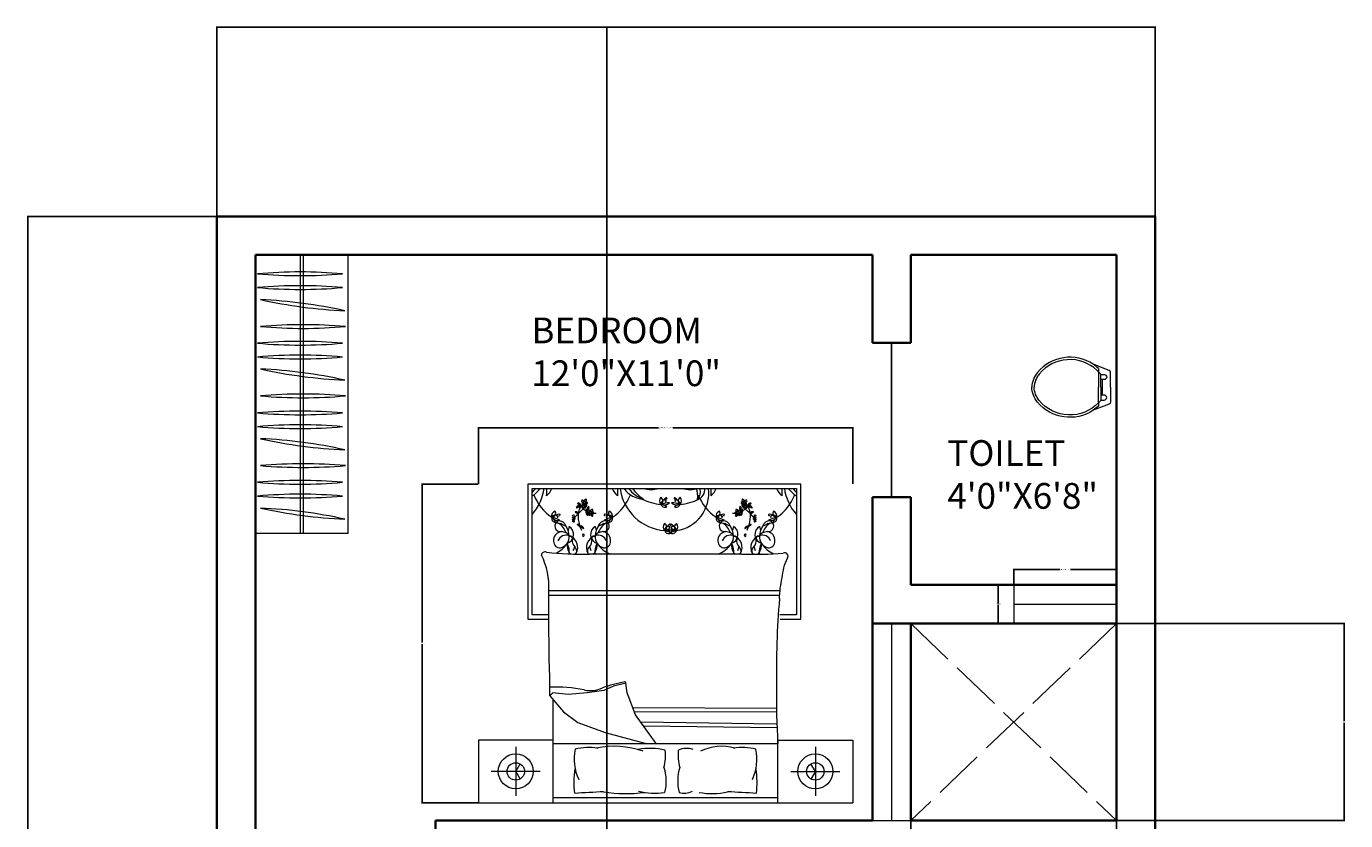
# Model space of a CAD drawing. Units: inches. Extents: x -16 to 587, y -783 to 64.
# Tile 14 of 14: x 279 to 587, y -122 to 64. Entities that reach past the tile are written whole.
import ezdxf

# ---------------------------------------------------------------- set-up
doc = ezdxf.new("R2010")
doc.units = ezdxf.units.IN
doc.header["$MEASUREMENT"] = 0
doc.linetypes.add('ACAD_ISO02W100', pattern=[15, 12, -3])
for name, color, linetype, lineweight in [('A-ANNO-DIMS', 2, 'Continuous', 18), ('A-AREA-IDEN', 7, 'Continuous', 18), ('A-DOOR', 3, 'Continuous', 25), ('A-FLOR-FIXT', 9, 'Continuous', 18), ('A-FLOR-OPEN', 8, 'ACAD_ISO02W100', 13), ('A-FURN', 8, 'Continuous', 18), ('A-GLAZ', 4, 'Continuous', 18), ('A-WALL', 7, 'Continuous', 35)]:
    doc.layers.add(name, color=color, linetype=linetype, lineweight=lineweight)
doc.styles.get("Standard").update_dxf_attribs({"font": 'arial.ttf'})
doc.dimstyles.get("Standard").update_dxf_attribs({"dimtxt": 0.18, "dimasz": 0.18, "dimexe": 0.18, "dimexo": 0.0625, "dimgap": 0.09, "dimtad": 0, "dimtih": 1, "dimtoh": 1, "dimdec": 0, "dimzin": 0, "dimdsep": 46, "dimlunit": 3, "dimtxsty": 'Standard', "dimcen": 0.09, "dimadec": 0, "dimazin": 0, "dimtfac": 1, "dimtdec": 0, "dimtofl": 0, "dimtmove": 0, "dimatfit": 3, "dimfxl": 1, "dimtolj": 1, "dimtzin": 0, "dimarcsym": 0})

# ---------------------------------------------------------------- blocks, each defined once
blk = doc.blocks.new('BED-DOUBLE-LARGE')
for p, q in [((11.54, 74.35), (11.54, 42.86)), ((75.28, 74.35), (11.54, 74.35)), ((75.28, 42.86), (75.28, 74.35)), ((12.55, 73.34), (74.26, 73.34)), ((12.55, 43.87), (12.55, 73.34)), ((74.26, 73.34), (74.26, 43.87)), ((21.17, 64.47), (20.98, 63.49)), ((27.28, 64.47), (27.47, 63.49)), ((59.54, 64.47), (59.35, 63.49)), ((65.65, 64.47), (65.84, 63.49)), ((61.46, 57.99), (25.97, 57.99)), ((70.42, 49.4), (16.48, 49.4)), ((70.34, 48.31), (16.48, 48.31)), ((16.48, 43.87), (12.55, 43.87)), ((74.26, 43.87), (70.41, 43.87)), ((11.54, 42.86), (16.49, 42.86)), ((70.43, 42.86), (75.28, 42.86)), ((34.41, 27.92), (31.58, 27.21)), ((34.77, 25.62), (34.41, 27.92)), ((17.41, 25.62), (16.7, 24.91)), ((16.7, 24.91), (19.89, 21.19)), ((20.95, 25.26), (17.41, 25.62)), ((25.38, 25.62), (20.95, 25.26)), ((29.28, 26.15), (25.38, 25.62)), ((31.58, 27.21), (29.28, 26.15)), ((36.71, 20.49), (34.77, 25.62)), ((17.49, 0), (17.49, 24)), ((69.63, 22), (36.09, 22.13)), ((19.89, 21.19), (23.25, 18.72)), ((23.25, 18.72), (29.63, 16.41)), ((69.63, 21.1), (36.43, 21.23)), ((41.5, 13.82), (36.71, 20.49)), ((69.67, 18.35), (37.93, 18.79)), ((29.63, 16.41), (39.16, 13.82)), ((69.71, 17.45), (38.58, 17.88)), ((8.74, 13), (8.74, 1.57)), ((17.49, 13.82), (69.94, 13.82)), ((78.68, 13), (78.68, 1.57)), ((14.46, 7.29), (3.03, 7.29)), ((72.97, 7.29), (84.4, 7.29)), ((0, 0), (87.43, 0)), ((69.94, 1.12), (17.49, 1.12))]:
    blk.add_line(p, q)
for points in [[(16.52, 32.91, -0.001242), (16.48, 49.5, 0.127202), (14.73, 57.77)], [(70.32, 47.62, -0.056112), (70.95, 52.43, -0.095341), (72.18, 57.07)], [(22.51, 2.18, -0.074897), (22.61, 7.89, 0.472817)], [(43.3, 8.21, -0.14099), (43.48, 2.38, -0.235245)], [(47.04, 8.21, 0.14099), (46.86, 2.38, 0.235245)], [(64.92, 2.18, 0.074897), (64.81, 7.89, -0.472817)]]:
    blk.add_lwpolyline(points, format="xyb")
for points in [[(17.49, 14.57), (0, 14.57), (0, 0)], [(69.94, 0), (69.94, 14.57), (87.43, 14.57), (87.43, 0)], [(8.74, 7.29), (9.76, 9.05)], [(8.74, 7.29), (9.76, 5.52)], [(78.68, 7.29), (77.66, 9.05)], [(78.68, 7.29), (77.66, 5.52)]]:
    blk.add_lwpolyline(points)
for centre, radius in [((24.76, 69.99), 0.223), ((26.22, 67.64), 0.223), ((60.6, 67.64), 0.223), ((62.05, 69.99), 0.223), ((8.74, 7.29), 4.08), ((8.74, 7.29), 2.04), ((78.68, 7.29), 4.08), ((78.68, 7.29), 2.04)]:
    blk.add_circle(centre, radius)
for centre, radius, start, end in [((7.78, 77.44), 6.93, 313.5186, 323.6964), ((9.78, 76.41), 5.56, 299.8884, 326.5383), ((4.05, 74.88), 11.42, 318.1144, 352.255), ((23.59, 76.01), 11.42, 201.4092, 235.6135), ((12.9, 75.12), 4.64, 311.0454, 337.4453), ((0.18, 72.62), 15.8, 356.3481, 2.5919), ((35.55, 75.12), 4.64, 202.5547, 228.9546), ((24.86, 76.01), 11.42, 304.3865, 338.5908), ((48.27, 72.62), 15.8, 177.4081, 183.6519), ((44.39, 74.88), 11.42, 187.745, 265.5377), ((38.67, 76.41), 5.56, 213.4617, 268.728), ((40.67, 77.44), 6.93, 216.3036, 252.1496), ((44.31, 79.39), 10.31, 215.947, 235.9877), ((43.52, 80.99), 11.42, 242.5854, 265.5377), ((40.33, 79.34), 6.28, 252.9798, 286.4569), ((42.81, 82.58), 9.28, 264.3643, 265.6213), ((47.7, 88.94), 16.59, 250.0972, 250.2783), ((43.57, 70.46), 1.27, 140.8855, 222.2127), ((42.13, 70.42), 0.953, 301.6373, 61.4609), ((45.36, 68.67), 2.89, 121.989, 161.0841), ((43.91, 71), 0.142, 288.4408, 121.989), ((43.93, 70.93), 0.0689, 171.9833, 288.4408), ((45.82, 71), 0.142, 58.011, 251.5592), ((45.8, 70.93), 0.0689, 251.5592, 8.0167), ((44.37, 68.67), 2.89, 18.9159, 58.011), ((44.97, 72.24), 8.84, 278.1803, 7.1364), ((47.6, 70.42), 0.953, 118.5391, 238.3627), ((46.16, 70.46), 1.27, 317.7873, 39.1145), ((46.21, 80.99), 11.42, 274.4623, 297.4146), ((49.41, 79.34), 6.28, 253.5431, 287.0202), ((46.92, 82.58), 9.28, 274.3787, 275.6357), ((42.03, 88.94), 16.59, 289.7217, 289.9028), ((46.11, 71.43), 5.11, 353.3805, 21.883), ((50.8, 72.86), 2.05, 280.9261, 13.6102), ((49.26, 72.57), 2.59, 318.0951, 17.1391), ((61.96, 76.01), 11.42, 201.4092, 235.6135), ((38.55, 72.62), 15.8, 356.3481, 2.5919), ((51.27, 75.12), 4.64, 311.0454, 337.4453), ((73.92, 75.12), 4.64, 202.5547, 228.9546), ((63.23, 76.01), 11.42, 304.3865, 338.5908), ((86.64, 72.62), 15.8, 177.4081, 183.6519), ((82.76, 74.88), 11.42, 187.745, 221.8856), ((77.04, 76.41), 5.56, 213.4617, 240.1116), ((79.04, 77.44), 6.93, 216.3036, 226.4814), ((18.37, 66.85), 1.27, 110.9613, 192.2885), ((17.11, 67.54), 0.953, 271.7131, 31.5367), ((22.65, 65.38), 2.47, 82.8698, 91.6736), ((22.99, 68.05), 0.459, 205.5379, 258.6744), ((22.33, 66.49), 1.38, 59.344, 79.7412), ((23.14, 68.85), 0.249, 123.0979, 213.1364), ((23.57, 68.49), 0.673, 92.3172, 160.5201), ((26.65, 63.38), 6.5, 121.1156, 124.8118), ((22.89, 67.42), 0.42, 355.7131, 81.6568), ((23.49, 68.75), 0.58, 82.6008, 147.1845), ((23.33, 69.66), 0.249, 55.6077, 145.6462), ((23.16, 69.13), 0.673, 21.7087, 93.0299), ((19.61, 64.33), 6.5, 53.6254, 57.3216), ((23.42, 68.72), 0.257, 45.7354, 121.1156), ((26.93, 67.08), 3.63, 150.7959, 175.244), ((32.15, 59.35), 11.95, 127.8256, 137.7588), ((23.36, 69.3), 0.58, 342.8042, 79.6943), ((23.31, 69.36), 0.257, 338.2452, 53.6254), ((23.73, 69.19), 0.194, 158.2452, 340.6395), ((23.74, 69.05), 0.194, 225.7354, 48.1297), ((27.39, 70.82), 3.88, 201.7087, 206.2181), ((24.3, 68.17), 1.01, 40.9365, 112.7695), ((23.96, 68.51), 0.597, 49.3812, 95.5456), ((26.93, 67.08), 3.63, 137.5083, 145.9967), ((24.4, 68.75), 0.617, 61.1838, 141.6792), ((27.3, 71.9), 4.35, 220.182, 239.456), ((24.3, 70.41), 0.221, 134.3732, 211.9501), ((24.7, 70.66), 0.702, 211.9501, 255.2442), ((24.31, 70.16), 0.439, 8.5614, 112.5914), ((24.52, 69.68), 0.304, 88.5719, 233.8954), ((24.48, 69.6), 0.218, 228.2946, 6.2474), ((24.82, 69.51), 0.718, 229.3812, 289.9959), ((24.43, 70.18), 0.147, 352.868, 97.094), ((24.28, 69.86), 0.306, 298.8493, 359.9355), ((24.35, 69.6), 0.35, 4.2123, 48.1587), ((25.07, 70.4), 0.368, 100.9597, 208.7804), ((25.07, 69.64), 0.371, 183.635, 258.4363), ((24.36, 68.63), 0.737, 15.6484, 62.2957), ((25.02, 69.78), 0.213, 178.1325, 268.8919), ((25.46, 69.91), 0.676, 132.3896, 156.5724), ((25.17, 69.83), 0.364, 42.3208, 130.2111), ((25.25, 70.21), 0.46, 226.3462, 279.6513), ((24.77, 69.35), 0.535, 7.4968, 71.2737), ((24.76, 70.6), 0.517, 291.6382, 4.947), ((25.16, 70.68), 0.729, 254.2829, 276.9148), ((25.1, 70.63), 0.171, 4.947, 127.5263), ((25.14, 69.38), 0.172, 215.0752, 14.7644), ((24.78, 69.11), 1.01, 287.889, 359.722), ((24.75, 68.64), 0.597, 305.1128, 351.2773), ((25.06, 67.54), 0.617, 3.8774, 87.1501), ((24.62, 67.78), 0.597, 352.0748, 38.2393), ((24.52, 67.31), 1.01, 343.6301, 55.4631), ((25.23, 68.74), 0.617, 271.4625, 339.4747), ((25.29, 69.94), 0.192, 279.6513, 42.3208), ((26.05, 68.44), 0.718, 110.6625, 171.2773), ((25.75, 68.06), 0.221, 134.3732, 211.9501), ((27.3, 71.9), 4.35, 246.1523, 246.9499), ((26.16, 68.32), 0.702, 211.9501, 255.2442), ((25.77, 67.81), 0.439, 8.5614, 112.5914), ((25.13, 68.8), 0.737, 338.3627, 25.0101), ((25.89, 67.83), 0.147, 352.868, 97.094), ((26.52, 68.05), 0.368, 100.9597, 208.7804), ((26.92, 67.57), 0.676, 132.3896, 156.5724), ((26.62, 67.48), 0.364, 42.3208, 130.2111), ((26.21, 68.25), 0.517, 291.6382, 4.947), ((26.56, 68.28), 0.171, 4.947, 127.5263), ((31.34, 67.54), 0.953, 148.4633, 268.2869), ((30.07, 66.85), 1.27, 347.7115, 69.0387), ((43.56, 69.65), 0.934, 76.148, 182.2415), ((45.02, 61.99), 7.99, 92.7418, 107.407), ((43.37, 71.25), 1.8, 245.6899, 314.4589), ((42.58, 67.66), 1.95, 44.6273, 88.5415), ((43.54, 69.87), 0.946, 196.1963, 296.9726), ((43.76, 70.43), 0.123, 140.0755, 76.148), ((44.71, 61.99), 7.99, 72.593, 87.2582), ((46.36, 71.25), 1.8, 225.5411, 294.3101), ((47.15, 67.66), 1.95, 91.4585, 135.3727), ((46.19, 69.87), 0.946, 243.0274, 343.8037), ((45.96, 70.39), 0.0744, 103.9791, 39.8091), ((46.17, 69.65), 0.934, 357.7585, 103.852), ((56.75, 66.85), 1.27, 110.9613, 192.2885), ((55.48, 67.54), 0.953, 271.7131, 31.5367), ((60.2, 67.48), 0.364, 49.7889, 137.6792), ((60.26, 68.28), 0.171, 52.4737, 175.053), ((60.61, 68.25), 0.517, 175.053, 248.3618), ((59.9, 67.57), 0.676, 23.4276, 47.6104), ((60.3, 68.05), 0.368, 331.2196, 79.0403), ((61.05, 67.81), 0.439, 67.4086, 171.4386), ((60.93, 67.83), 0.147, 82.906, 187.132), ((60.66, 68.32), 0.702, 284.7558, 328.0499), ((61.69, 68.8), 0.737, 154.9899, 201.6373), ((61.58, 68.74), 0.617, 200.5253, 268.5375), ((62.04, 69.11), 1.01, 180.278, 252.111), ((60.77, 68.44), 0.718, 8.7227, 69.3375), ((61.76, 67.54), 0.617, 92.8499, 176.1226), ((61.07, 68.06), 0.221, 328.0499, 45.6268), ((59.52, 71.9), 4.35, 293.0501, 293.8477), ((62.3, 67.31), 1.01, 124.5369, 196.3699), ((61.52, 69.94), 0.192, 137.6792, 260.3487), ((61.65, 69.83), 0.364, 49.7889, 137.6792), ((62.07, 68.64), 0.597, 188.7227, 234.8872), ((61.57, 70.21), 0.46, 260.3487, 313.6538), ((62.05, 69.35), 0.535, 108.7263, 172.5032), ((61.68, 69.38), 0.172, 165.2356, 324.9248), ((61.72, 70.63), 0.171, 52.4737, 175.053), ((62.06, 70.6), 0.517, 175.053, 248.3618), ((61.66, 70.68), 0.729, 263.0852, 285.7171), ((62.2, 67.78), 0.597, 141.7607, 187.9252), ((59.52, 71.9), 4.35, 300.544, 319.818), ((62.46, 68.63), 0.737, 117.7043, 164.3516), ((62.52, 68.17), 1.01, 67.2305, 139.0635), ((62, 69.51), 0.718, 250.0041, 310.6188), ((61.8, 69.78), 0.213, 271.1081, 1.8675), ((61.35, 69.91), 0.676, 23.4276, 47.6104), ((61.75, 70.4), 0.368, 331.2196, 79.0403), ((61.75, 69.64), 0.371, 281.5637, 356.365), ((54.66, 59.35), 11.95, 42.2412, 52.1744), ((62.51, 70.16), 0.439, 67.4086, 171.4386), ((62.47, 69.6), 0.35, 131.8413, 175.7877), ((62.33, 69.6), 0.218, 173.7526, 311.7054), ((62.42, 68.75), 0.617, 38.3208, 118.8162), ((62.54, 69.86), 0.306, 180.0645, 241.1507), ((62.38, 70.18), 0.147, 82.906, 187.132), ((62.11, 70.66), 0.702, 284.7558, 328.0499), ((62.3, 69.68), 0.304, 306.1046, 91.4281), ((62.85, 68.51), 0.597, 84.4544, 130.6188), ((59.89, 67.08), 3.63, 34.0033, 42.4917), ((62.52, 70.41), 0.221, 328.0499, 45.6268), ((63.45, 69.3), 0.58, 100.3057, 197.1958), ((63.08, 69.05), 0.194, 131.8703, 314.2646), ((63.08, 69.19), 0.194, 199.3605, 21.7548), ((59.43, 70.82), 3.88, 333.7819, 338.2913), ((63.66, 69.13), 0.673, 86.9701, 158.2913), ((59.89, 67.08), 3.63, 4.756, 29.2041), ((63.4, 68.72), 0.257, 58.8844, 134.2646), ((63.5, 69.36), 0.257, 126.3746, 201.7548), ((63.32, 68.75), 0.58, 32.8155, 97.3992), ((63.25, 68.49), 0.673, 19.4799, 87.6828), ((63.49, 69.66), 0.249, 34.3538, 124.3923), ((67.21, 64.33), 6.5, 122.6784, 126.3746), ((63.93, 67.42), 0.42, 98.3432, 184.2869), ((60.17, 63.38), 6.5, 55.1882, 58.8844), ((64.49, 66.49), 1.38, 100.2588, 120.656), ((63.67, 68.85), 0.249, 326.8636, 56.9021), ((64.17, 65.38), 2.47, 88.3264, 97.1302), ((63.83, 68.05), 0.459, 281.3256, 334.4621), ((69.71, 67.54), 0.953, 148.4633, 268.2869), ((68.44, 66.85), 1.27, 347.7115, 69.0387), ((18.06, 66.36), 0.946, 166.272, 267.0484), ((19.04, 64.41), 2.89, 92.0648, 131.1598), ((17.96, 66.15), 0.934, 46.2238, 152.3173), ((15.41, 58.79), 7.99, 62.8176, 77.4827), ((18.6, 67.64), 1.8, 215.7657, 284.5347), ((16.12, 64.92), 1.95, 14.7031, 58.6173), ((19.17, 64.55), 1.31, 109.1312, 279.736), ((18.9, 65.97), 0.804, 216.7319, 296.0245), ((18.53, 66.74), 0.123, 110.2817, 46.2238), ((16.57, 61.66), 4.13, 18.2955, 58.7386), ((18.85, 64.15), 1.64, 15.6955, 94.031), ((18.92, 67.08), 0.0689, 142.0591, 258.5166), ((18.94, 67.15), 0.142, 258.5166, 92.0648), ((20.62, 66.33), 1.75, 218.4175, 263.8338), ((22.21, 66.73), 0.368, 100.9597, 142.2379), ((21.9, 66.32), 0.223, 273.2768, 86.7232), ((22.21, 65.97), 0.371, 217.3642, 258.4363), ((22.16, 66.11), 0.213, 178.1325, 268.8919), ((22.6, 66.24), 0.676, 132.3896, 156.5724), ((22.31, 66.16), 0.364, 42.3208, 130.2111), ((22.39, 66.54), 0.46, 226.3462, 279.6513), ((21.91, 65.68), 0.535, 7.4968, 71.2737), ((21.9, 66.93), 0.517, 291.6382, 4.947), ((22.3, 67.01), 0.729, 254.2829, 276.9148), ((22.24, 66.96), 0.171, 4.947, 127.5263), ((22.28, 65.71), 0.172, 215.0752, 14.7644), ((17.25, 73.06), 8.3, 307.9541, 316.8459), ((22.43, 66.27), 0.192, 279.6513, 42.3208), ((22.03, 66.49), 1.4, 43.6929, 51.7899), ((22.66, 67.05), 0.733, 27.3659, 59.344), ((23.21, 67.53), 0.178, 202.5583, 304.2343), ((23.17, 62.44), 2.47, 82.8698, 91.6736), ((23.51, 65.1), 0.459, 205.5379, 258.6744), ((22.85, 63.55), 1.38, 59.344, 79.7412), ((30.53, 66.9), 7.24, 176.1723, 196.4158), ((23.41, 64.47), 0.42, 355.7131, 81.6568), ((23.18, 64.11), 0.733, 27.3659, 59.344), ((25.92, 67.6), 0.718, 172.0748, 232.6895), ((24.94, 67.52), 0.737, 318.342, 4.9894), ((25.97, 67.33), 0.304, 88.5719, 233.8954), ((25.94, 67.25), 0.218, 228.2946, 6.2474), ((25.73, 67.51), 0.306, 298.8493, 359.9355), ((25.81, 67.25), 0.35, 4.2123, 48.1587), ((26.53, 67.3), 0.371, 183.635, 258.4363), ((26.48, 67.43), 0.213, 178.1325, 268.8919), ((26.7, 67.86), 0.46, 226.3462, 279.6513), ((26.23, 67.01), 0.535, 7.4968, 71.2737), ((26.62, 68.34), 0.729, 254.2829, 276.9148), ((26.59, 67.03), 0.172, 215.0752, 14.7644), ((26.75, 67.59), 0.192, 279.6513, 42.3208), ((27.3, 71.9), 4.35, 265.2415, 272.8929), ((31.88, 61.66), 4.13, 121.2614, 161.7045), ((29.59, 64.15), 1.64, 85.969, 164.3045), ((27.83, 66.33), 1.75, 276.1662, 321.5825), ((29.28, 64.55), 1.31, 260.264, 70.8688), ((29.55, 65.97), 0.804, 243.9755, 323.2681), ((29.51, 67.15), 0.142, 87.9352, 281.4834), ((29.84, 67.64), 1.8, 255.4653, 324.2343), ((33.04, 58.79), 7.99, 102.5173, 117.1824), ((29.41, 64.41), 2.89, 48.8402, 87.9352), ((29.52, 67.08), 0.0689, 281.4834, 37.9409), ((30.48, 66.15), 0.934, 27.6827, 133.7762), ((29.94, 66.69), 0.0744, 133.7729, 69.7333), ((30.39, 66.36), 0.946, 272.9516, 13.728), ((32.32, 64.92), 1.95, 121.3827, 165.2969), ((44.44, 64.35), 1.27, 140.8855, 222.2127), ((43.01, 64.31), 0.953, 301.6373, 61.4609), ((46.24, 62.56), 2.89, 121.989, 161.0841), ((44.78, 64.89), 0.142, 288.4408, 121.989), ((44.81, 64.82), 0.0689, 171.9833, 288.4408), ((44.95, 64.89), 0.142, 58.011, 251.5592), ((44.93, 64.82), 0.0689, 251.5592, 8.0167), ((43.5, 62.56), 2.89, 18.9159, 58.011), ((46.73, 64.31), 0.953, 118.5391, 238.3627), ((45.29, 64.35), 1.27, 317.7873, 39.1145), ((56.43, 66.36), 0.946, 166.272, 267.0484), ((57.41, 64.41), 2.89, 92.0648, 131.1598), ((56.34, 66.15), 0.934, 46.2238, 152.3173), ((54.49, 64.92), 1.95, 14.7031, 58.6173), ((56.97, 67.64), 1.8, 215.7657, 284.5347), ((53.78, 58.79), 7.99, 62.8176, 77.4827), ((57.54, 64.55), 1.31, 109.1312, 279.736), ((57.27, 65.97), 0.804, 216.7319, 296.0245), ((56.9, 66.74), 0.123, 110.2817, 46.2238), ((54.94, 61.66), 4.13, 18.2955, 58.7386), ((57.22, 64.15), 1.64, 15.6955, 94.031), ((57.3, 67.08), 0.0689, 142.0591, 258.5166), ((57.31, 67.15), 0.142, 258.5166, 92.0648), ((58.99, 66.33), 1.75, 218.4175, 263.8338), ((59.52, 71.9), 4.35, 267.1071, 274.7585), ((60.07, 67.59), 0.192, 137.6792, 260.3487), ((60.11, 67.86), 0.46, 260.3487, 313.6538), ((60.22, 67.03), 0.172, 165.2356, 324.9248), ((60.59, 67.01), 0.535, 108.7263, 172.5032), ((60.2, 68.34), 0.729, 263.0852, 285.7171), ((60.34, 67.43), 0.213, 271.1081, 1.8675), ((60.29, 67.3), 0.371, 281.5637, 356.365), ((61.01, 67.25), 0.35, 131.8413, 175.7877), ((60.88, 67.25), 0.218, 173.7526, 311.7054), ((61.08, 67.51), 0.306, 180.0645, 241.1507), ((60.84, 67.33), 0.304, 306.1046, 91.4281), ((61.88, 67.52), 0.737, 175.0106, 221.658), ((60.89, 67.6), 0.718, 307.3105, 7.9252), ((63.41, 64.47), 0.42, 98.3432, 184.2869), ((63.64, 64.11), 0.733, 120.656, 152.6341), ((56.28, 66.9), 7.24, 343.5842, 3.8277), ((63.97, 63.55), 1.38, 100.2588, 120.656), ((63.65, 62.44), 2.47, 88.3264, 97.1302), ((63.31, 65.1), 0.459, 281.3256, 334.4621), ((64.16, 67.05), 0.733, 120.656, 152.6341), ((63.61, 67.53), 0.178, 235.7657, 337.4417), ((69.56, 73.06), 8.3, 223.1541, 232.0459), ((64.79, 66.49), 1.4, 128.2101, 136.3071), ((64.38, 66.27), 0.192, 137.6792, 260.3487), ((64.51, 66.16), 0.364, 49.7889, 137.6792), ((64.43, 66.54), 0.46, 260.3487, 313.6538), ((64.9, 65.68), 0.535, 108.7263, 172.5032), ((64.54, 65.71), 0.172, 165.2356, 324.9248), ((64.58, 66.96), 0.171, 52.4737, 175.053), ((64.92, 66.93), 0.517, 175.053, 248.3618), ((64.52, 67.01), 0.729, 263.0852, 285.7171), ((64.66, 66.11), 0.213, 271.1081, 1.8675), ((64.21, 66.24), 0.676, 23.4276, 47.6104), ((64.61, 66.73), 0.368, 37.7621, 79.0403), ((64.61, 65.97), 0.371, 281.5637, 322.6358), ((64.91, 66.32), 0.223, 93.2768, 266.7232), ((70.25, 61.66), 4.13, 121.2614, 161.7045), ((67.96, 64.15), 1.64, 85.969, 164.3045), ((66.2, 66.33), 1.75, 276.1662, 321.5825), ((67.65, 64.55), 1.31, 260.264, 70.8688), ((67.92, 65.97), 0.804, 243.9755, 323.2681), ((67.88, 67.15), 0.142, 87.9352, 281.4834), ((71.41, 58.79), 7.99, 102.5173, 117.1824), ((68.22, 67.64), 1.8, 255.4653, 324.2343), ((67.78, 64.41), 2.89, 48.8402, 87.9352), ((67.89, 67.08), 0.0689, 281.4834, 37.9409), ((68.85, 66.15), 0.934, 27.6827, 133.7762), ((68.31, 66.69), 0.0744, 133.7729, 69.7333), ((70.7, 64.92), 1.95, 121.3827, 165.2969), ((68.76, 66.36), 0.946, 272.9516, 13.728), ((19.65, 61.18), 2.09, 97.1143, 185.0551), ((20.47, 60.39), 2.03, 68.5779, 158.4181), ((18.59, 62.06), 2.63, 283.079, 4.7067), ((19.29, 60.71), 2.54, 35.9599, 87.6409), ((16.53, 61.99), 4.69, 3.4924, 33.7117), ((20.08, 62.59), 2.17, 286.8663, 60.0915), ((24.06, 60.21), 3.37, 143.6555, 147.2989), ((21.46, 61.68), 0.543, 344.8529, 102.6959), ((20.42, 59.58), 2.79, 330.8249, 70.7178), ((22.55, 63.55), 1.4, 43.6929, 51.7899), ((23.73, 64.59), 0.178, 202.5583, 304.2343), ((30.53, 66.9), 7.24, 200.1059, 206.9968), ((24.06, 64.09), 0.42, 36.5232, 122.4668), ((23.84, 63.71), 0.733, 58.836, 90.8141), ((24.01, 64.42), 0.178, 173.9457, 275.6216), ((23.65, 62.89), 1.4, 66.3901, 74.4871), ((24.57, 64.47), 0.459, 219.5056, 272.6421), ((23.5, 63.15), 1.38, 38.4388, 58.836), ((24.47, 62.5), 0.169, 79.5616, 257.2949), ((22.38, 62.91), 2.47, 26.5064, 35.3102), ((24.46, 62.4), 0.274, 259.5864, 79.5616), ((28.03, 59.58), 2.79, 109.2822, 209.1751), ((28.36, 62.59), 2.17, 119.9085, 253.1337), ((26.99, 61.68), 0.543, 77.3041, 195.1471), ((29.16, 60.71), 2.54, 92.3591, 144.0401), ((24.39, 60.21), 3.37, 32.7011, 36.3445), ((29.86, 62.06), 2.63, 175.2933, 256.921), ((31.92, 61.99), 4.69, 146.2883, 176.5076), ((27.98, 60.39), 2.03, 21.5819, 111.4221), ((28.8, 61.18), 2.09, 354.9449, 82.8857), ((44.44, 63.53), 0.934, 76.148, 182.2415), ((44.25, 65.14), 1.8, 245.6899, 314.4589), ((45.89, 55.87), 7.99, 92.7418, 107.407), ((44.41, 63.76), 0.946, 196.1963, 296.9726), ((43.46, 61.55), 1.95, 44.6273, 88.5415), ((45.48, 65.14), 1.8, 225.5411, 294.3101), ((43.84, 55.87), 7.99, 72.593, 87.2582), ((44.63, 64.32), 0.123, 140.0755, 76.148), ((45.32, 63.76), 0.946, 243.0274, 343.8037), ((46.28, 61.55), 1.95, 91.4585, 135.3727), ((45.09, 64.27), 0.0744, 103.9791, 39.8091), ((45.29, 63.53), 0.934, 357.7585, 103.852), ((58.02, 61.18), 2.09, 97.1143, 185.0551), ((58.84, 60.39), 2.03, 68.5779, 158.4181), ((56.96, 62.06), 2.63, 283.079, 4.7067), ((57.66, 60.71), 2.54, 35.9599, 87.6409), ((54.9, 61.99), 4.69, 3.4924, 33.7117), ((58.46, 62.59), 2.17, 286.8663, 60.0915), ((62.43, 60.21), 3.37, 143.6555, 147.2989), ((59.83, 61.68), 0.543, 344.8529, 102.6959), ((58.79, 59.58), 2.79, 330.8249, 70.7178), ((62.36, 62.4), 0.274, 100.4384, 280.4136), ((63.31, 63.15), 1.38, 121.164, 141.5612), ((64.44, 62.91), 2.47, 144.6898, 153.4936), ((62.25, 64.47), 0.459, 267.3579, 320.4944), ((62.34, 62.5), 0.169, 282.7051, 100.4384), ((62.76, 64.09), 0.42, 57.5332, 143.4768), ((62.98, 63.71), 0.733, 89.1859, 121.164), ((63.17, 62.89), 1.4, 105.5129, 113.6099), ((56.28, 66.9), 7.24, 333.0032, 339.8941), ((62.81, 64.42), 0.178, 264.3784, 6.0543), ((63.09, 64.59), 0.178, 235.7657, 337.4417), ((64.27, 63.55), 1.4, 128.2101, 136.3071), ((66.4, 59.58), 2.79, 109.2822, 209.1751), ((66.73, 62.59), 2.17, 119.9085, 253.1337), ((65.36, 61.68), 0.543, 77.3041, 195.1471), ((67.53, 60.71), 2.54, 92.3591, 144.0401), ((62.76, 60.21), 3.37, 32.7011, 36.3445), ((68.23, 62.06), 2.63, 175.2933, 256.921), ((70.29, 61.99), 4.69, 146.2883, 176.5076), ((66.35, 60.39), 2.03, 21.5819, 111.4221), ((67.17, 61.18), 2.09, 354.9449, 82.8857), ((15.53, 57.71), 0.807, 62.6588, 176.02), ((19.04, 60.97), 1.48, 178.9462, 275.5144), ((15.19, 64.15), 6.62, 296.7003, 326.3329), ((24.06, 60.21), 3.37, 175.2696, 214.215), ((17.62, 58.64), 3.62, 350.8446, 31.1782), ((23.71, 61.07), 1.79, 164.8529, 228.4347), ((20, 60.08), 2.51, 330.0851, 352.564), ((21.66, 58.75), 1.31, 336.1646, 48.4347), ((26.79, 58.75), 1.31, 131.5653, 203.8354), ((24.73, 61.07), 1.79, 311.5653, 15.1471), ((28.45, 60.08), 2.51, 187.436, 209.9149), ((24.39, 60.21), 3.37, 325.785, 4.7304), ((30.83, 58.64), 3.62, 148.8218, 190.2867), ((33.26, 64.15), 6.62, 213.6671, 248.5059), ((29.4, 60.97), 1.48, 264.4856, 1.0538), ((57.41, 60.97), 1.48, 178.9462, 275.5144), ((53.56, 64.15), 6.62, 291.4941, 326.3329), ((62.43, 60.21), 3.37, 175.2696, 214.215), ((55.99, 58.64), 3.62, 349.7133, 31.1782), ((62.09, 61.07), 1.79, 164.8529, 228.4347), ((58.37, 60.08), 2.51, 330.0851, 352.564), ((60.03, 58.75), 1.31, 336.1646, 48.4347), ((65.16, 58.75), 1.31, 131.5653, 203.8354), ((63.1, 61.07), 1.79, 311.5653, 15.1471), ((66.82, 60.08), 2.51, 187.436, 209.9149), ((62.76, 60.21), 3.37, 325.785, 4.7304), ((69.2, 58.64), 3.62, 148.8218, 190.751), ((71.63, 64.15), 6.62, 213.6671, 246.3547), ((67.77, 60.97), 1.48, 264.4856, 1.0538), ((24.92, 148.99), 91.01, 264.3113, 270.6567), ((22.1, 58.96), 1.05, 217.675, 239.9707), ((22.1, 58.96), 1.05, 296.442, 315.5483), ((26.34, 58.96), 1.05, 224.4517, 246.771), ((26.34, 58.96), 1.05, 293.2856, 322.325), ((60.47, 58.96), 1.05, 217.675, 246.7144), ((60.47, 58.96), 1.05, 293.2856, 315.5483), ((64.14, 143.02), 85.07, 268.1965, 274.7598), ((64.72, 58.96), 1.05, 224.4517, 253.3657), ((64.72, 58.96), 1.05, 287.4186, 322.325), ((71.52, 57.51), 0.797, 326.1736, 113.4781), ((274.49, 30.21), 204.92, 175.1265, 180.8855), ((-63.46, 27.08), 80.19, 358.447, 4.1706), ((40.48, -5.12), 33.91, 100.6617, 109.8806), ((34.21, 27.99), 0.211, 340.2464, 91.1377), ((18.2, -6.05), 33, 78.6608, 92.5481), ((26.09, 33.28), 7.12, 258.6608, 293.7384), ((226.67, 24.5), 157.09, 179.0718, 183.9), ((33.65, 10.18), 11.27, 168.2417, 204.8684), ((25.63, 1.16), 11.72, 78.9631, 104.8961), ((31.79, -7.17), 20.32, 70.7385, 101.9603), ((40.02, -2.74), 15.42, 76.3762, 100.1383), ((48.65, 8.05), 4.63, 71.4593, 114.9817), ((56.75, 2.02), 11.13, 73.8254, 116.1239), ((61.8, 1.16), 11.72, 75.1039, 101.0369), ((53.78, 10.18), 11.27, 335.1316, 11.7583), ((33, 11.13), 10.71, 344.1707, 5.9871), ((57.34, 11.13), 10.71, 174.0129, 195.8293), ((70.7, -829.84), 833.41, 92.85022, 93.31479), ((34.49, 33.82), 31.71, 260.503, 277.7804), ((41.18, 17.79), 15.58, 256.04, 278.4751), ((48.06, 6.54), 4.32, 253.8974, 296.6563), ((54.54, 17.48), 15.37, 258.8159, 283.6573), ((16.73, -829.84), 833.41, 86.68521, 87.14978)]:
    blk.add_arc(centre, radius, start, end)
blk = doc.blocks.new('WARDROBE')
for p, q in [((0, 0), (0, 65.01)), ((21.67, 65.01), (0, 65.01)), ((10.47, 0), (10.47, 65.01)), ((11.19, 0), (11.19, 65.01)), ((21.67, 0), (21.67, 65.01)), ((21.67, 0), (0, 0))]:
    blk.add_line(p, q)
for centre, start, end in [((10.4, -52.98), 85.0028, 94.9972), ((10.4, 174.18), 265.0028, 274.9972), ((10.4, -56.19), 85.0028, 94.9972), ((10.4, 170.97), 265.0028, 274.9972), ((25.83, 165.89), 257.508, 267.5023), ((-3.8, -59.33), 77.508, 87.5023), ((11.1, -65.28), 85.0028, 94.9972), ((11.1, 161.88), 265.0028, 274.9972), ((10.4, -69.18), 85.0028, 94.9972), ((10.4, 157.98), 265.0028, 274.9972), ((10.4, -72.39), 85.0028, 94.9972), ((10.4, 154.77), 265.0028, 274.9972), ((25.83, 149.7), 257.508, 267.5023), ((-3.8, -75.52), 77.508, 87.5023), ((11.1, -81.47), 85.0028, 94.9972), ((11.1, 145.69), 265.0028, 274.9972), ((10.4, -85.44), 85.0028, 94.9972), ((10.4, 141.72), 265.0028, 274.9972), ((10.4, -88.65), 85.0028, 94.9972), ((10.4, 138.51), 265.0028, 274.9972), ((-3.8, -91.78), 77.508, 87.5023), ((25.83, 133.44), 257.508, 267.5023), ((11.1, -97.73), 85.0028, 94.9972), ((11.1, 129.43), 265.0028, 274.9972), ((10.4, -101.63), 85.0028, 94.9972), ((10.4, 125.53), 265.0028, 274.9972), ((10.4, -104.84), 85.0028, 94.9972), ((10.4, 122.32), 265.0028, 274.9972), ((-3.8, -107.97), 77.508, 87.5023), ((25.83, 117.25), 257.508, 267.5023)]:
    blk.add_arc(centre, 114.01, start, end)
blk = doc.blocks.new('WC-PLAN')
for p, q in [((15.58, 11.39), (15.58, 10.62)), ((15.58, 10.62), (15.58, 7.01)), ((15.58, 3.4), (15.58, 7.01)), ((15.58, 3.4), (15.58, 2.63))]:
    blk.add_line(p, q)
for points in [[(14.32, 12.39, 0.383919), (1.32, 10.46, 0.163732), (0, 7.01, 0.359733)], [(15.2, 10.99, 0.431639), (1.75, 10.11, 0.162618), (0.55, 7.01, 0.470877)], [(15.58, 11.39, 0.040937), (14.32, 12.39, 0.163732)], [(18.36, 7.01), (18.36, 10.52, 0.31031), (18.06, 10.95), (14.32, 12.39, 0.209071)], [(15.58, 10.62, 0.014165), (15.2, 10.99, 0.162618)], [(16.13, 9.99, 0.022712), (15.58, 10.62, 0.162618)], [(16.13, 7.01), (16.13, 9.99, 0.022712)], [(16.13, 9.99), (16.9, 9.99, -1), (16.9, 8.82), (16.5, 8.82)], [(14.32, 1.64, -0.383919), (1.32, 3.56, -0.163732), (0, 7.01, -0.359733)], [(15.58, 3.4, -0.448546), (1.75, 3.91, -0.162618), (0.55, 7.01, -0.470877)], [(18.36, 7.01), (18.36, 3.51, -0.31031), (18.06, 3.08), (14.32, 1.64, -0.209071)], [(16.13, 7.01), (16.13, 4.03, -0.476108)], [(16.13, 4.03, -0.022712), (15.58, 3.4, -0.162618)], [(16.13, 4.03), (16.9, 4.03, 1), (16.9, 5.21), (16.5, 5.21)], [(15.58, 2.63, -0.040937), (14.32, 1.64, -0.163732)]]:
    blk.add_lwpolyline(points, format="xyb")
for points in [[(16.5, 8.82), (16.13, 8.82)], [(16.5, 5.21), (16.5, 8.82)], [(16.5, 5.21), (16.13, 5.21)]]:
    blk.add_lwpolyline(points)
blk = doc.blocks.new('WIN-24')
for p, q in [((0, 9), (0, 0)), ((0, 9), (24, 9)), ((24, 9), (24, 0)), ((0, 4.5), (24, 4.5)), ((24, 0), (0, 0))]:
    blk.add_line(p, q)
blk = doc.blocks.new('WIN-48')
for p, q in [((0, 9), (0, 0)), ((48, 9), (0, 9)), ((48, 0), (48, 9)), ((0, 4.5), (48, 4.5)), ((0, 0), (48, 0))]:
    blk.add_line(p, q)
blk = doc.blocks.new('*D34')
at = {"layer": 'A-ANNO-DIMS', "color": 0, "lineweight": -2, "transparency": 16777216}
for p, q in [((384.81, -42.96), (384.81, -29.73)), ((384.99, -29.91), (426.84, -29.91)), ((472.06, -29.91), (430.21, -29.91)), ((472.24, -42.96), (472.24, -29.73))]:
    blk.add_line(p, q, dxfattribs=at)
at = {"layer": 'A-ANNO-DIMS', "color": 0, "transparency": 16777216}
for points in [[(384.99, -29.88), (384.99, -29.94), (384.81, -29.91)], [(472.06, -29.88), (472.06, -29.94), (472.24, -29.91)]]:
    blk.add_solid(points, dxfattribs=at)
at = {"layer": 'Defpoints', "color": 0, "transparency": 16777216}
for p in [(472.24, -29.91), (384.81, -43.02), (472.24, -43.02)]:
    blk.add_point(p, dxfattribs=at)
at = {"layer": 'A-ANNO-DIMS', "color": 0, "transparency": 16777216, "insert": (428.53, -29.91), "char_height": 0.18, "attachment_point": 5}
blk.add_mtext('\\A1;DOUBLE BED 7\'-3 1/2" TYP.', dxfattribs=at)
blk = doc.blocks.new('*D35')
at = {"layer": 'A-ANNO-DIMS', "color": 0, "lineweight": -2, "transparency": 16777216}
for p, q in [((384.75, -43.02), (371.52, -43.02)), ((371.7, -43.2), (371.7, -80.01)), ((371.7, -117.19), (371.7, -80.38)), ((384.75, -117.37), (371.52, -117.37))]:
    blk.add_line(p, q, dxfattribs=at)
at = {"layer": 'A-ANNO-DIMS', "color": 0, "transparency": 16777216}
for points in [[(371.67, -43.2), (371.73, -43.2), (371.7, -43.02)], [(371.67, -117.19), (371.73, -117.19), (371.7, -117.37)]]:
    blk.add_solid(points, dxfattribs=at)
at = {"layer": 'Defpoints', "color": 0, "transparency": 16777216}
for p in [(371.7, -43.02), (384.81, -43.02), (384.81, -117.37)]:
    blk.add_point(p, dxfattribs=at)
at = {"layer": 'A-ANNO-DIMS', "color": 0, "transparency": 16777216, "insert": (371.7, -80.19), "char_height": 0.18, "attachment_point": 5}
blk.add_mtext('\\A1;6\'-2 1/2" TYP.', dxfattribs=at)
blk = doc.blocks.new('*D42')
at = {"layer": 'A-ANNO-DIMS', "color": 0, "lineweight": -2, "transparency": 16777216}
for p, q in [((509.79, -66.49), (509.79, -62.77)), ((509.97, -62.95), (520.56, -62.95)), ((533.61, -62.95), (523.02, -62.95)), ((533.79, -66.49), (533.79, -62.77))]:
    blk.add_line(p, q, dxfattribs=at)
at = {"layer": 'A-ANNO-DIMS', "color": 0, "transparency": 16777216}
for points in [[(509.97, -62.92), (509.97, -62.98), (509.79, -62.95)], [(533.61, -62.92), (533.61, -62.98), (533.79, -62.95)]]:
    blk.add_solid(points, dxfattribs=at)
at = {"layer": 'Defpoints', "color": 0, "transparency": 16777216}
for p in [(533.79, -62.95), (509.79, -66.55), (533.79, -66.55)]:
    blk.add_point(p, dxfattribs=at)
at = {"layer": 'A-ANNO-DIMS', "color": 0, "transparency": 16777216, "insert": (521.79, -62.95), "char_height": 0.18, "attachment_point": 5}
blk.add_mtext('\\A1;WINDOW 2\'-0" TYP.', dxfattribs=at)
blk = doc.blocks.new('*D43')
at = {"layer": 'A-ANNO-DIMS', "color": 0, "lineweight": -2, "transparency": 16777216}
for p, q in [((509.73, -66.55), (506.01, -66.55)), ((506.19, -66.73), (506.19, -70.87)), ((506.19, -75.37), (506.19, -71.24)), ((509.73, -75.55), (506.01, -75.55))]:
    blk.add_line(p, q, dxfattribs=at)
at = {"layer": 'A-ANNO-DIMS', "color": 0, "transparency": 16777216}
for points in [[(506.16, -66.73), (506.22, -66.73), (506.19, -66.55)], [(506.16, -75.37), (506.22, -75.37), (506.19, -75.55)]]:
    blk.add_solid(points, dxfattribs=at)
at = {"layer": 'Defpoints', "color": 0, "transparency": 16777216}
for p in [(506.19, -66.55), (509.79, -66.55), (509.79, -75.55)]:
    blk.add_point(p, dxfattribs=at)
at = {"layer": 'A-ANNO-DIMS', "color": 0, "transparency": 16777216, "insert": (506.19, -71.05), "char_height": 0.18, "attachment_point": 5}
blk.add_mtext('\\A1;0\'-9" TYP.', dxfattribs=at)
blk = doc.blocks.new('*D52')
at = {"layer": 'A-ANNO-DIMS', "color": 0, "lineweight": -2, "transparency": 16777216}
for p, q in [((323.79, 19.51), (323.79, 63.78)), ((323.97, 63.6), (432.9, 63.6)), ((542.61, 63.6), (433.68, 63.6)), ((542.79, 19.51), (542.79, 63.78))]:
    blk.add_line(p, q, dxfattribs=at)
at = {"layer": 'A-ANNO-DIMS', "color": 0, "transparency": 16777216}
for points in [[(323.97, 63.63), (323.97, 63.57), (323.79, 63.6)], [(542.61, 63.63), (542.61, 63.57), (542.79, 63.6)]]:
    blk.add_solid(points, dxfattribs=at)
at = {"layer": 'Defpoints', "color": 0, "transparency": 16777216}
for p in [(542.79, 63.6), (323.79, 19.45), (542.79, 19.45)]:
    blk.add_point(p, dxfattribs=at)
at = {"layer": 'A-ANNO-DIMS', "color": 0, "transparency": 16777216, "insert": (433.29, 63.6), "char_height": 0.18, "attachment_point": 5}
blk.add_mtext('\\A1;18\'-3"', dxfattribs=at)
blk = doc.blocks.new('*D53')
at = {"layer": 'A-ANNO-DIMS', "color": 0, "lineweight": -2, "transparency": 16777216}
for p, q in [((323.73, 19.45), (279.46, 19.45)), ((279.64, 19.27), (279.64, -358.87)), ((279.64, -737.37), (279.64, -359.24)), ((323.73, -737.55), (279.46, -737.55))]:
    blk.add_line(p, q, dxfattribs=at)
at = {"layer": 'A-ANNO-DIMS', "color": 0, "transparency": 16777216}
for points in [[(279.61, 19.27), (279.67, 19.27), (279.64, 19.45)], [(279.61, -737.37), (279.67, -737.37), (279.64, -737.55)]]:
    blk.add_solid(points, dxfattribs=at)
at = {"layer": 'Defpoints', "color": 0, "transparency": 16777216}
for p in [(323.79, 19.45), (279.64, -737.55), (323.79, -737.55)]:
    blk.add_point(p, dxfattribs=at)
at = {"layer": 'A-ANNO-DIMS', "color": 0, "transparency": 16777216, "insert": (279.64, -359.05), "char_height": 0.18, "attachment_point": 5}
blk.add_mtext('\\A1;63\'-1"', dxfattribs=at)
blk = doc.blocks.new('*D54')
at = {"layer": 'A-ANNO-DIMS', "color": 0, "lineweight": -2, "transparency": 16777216}
for p, q in [((533.85, -75.55), (587.12, -75.55)), ((586.94, -75.73), (586.94, -98.37)), ((586.94, -121.37), (586.94, -98.74)), ((533.85, -121.55), (587.12, -121.55))]:
    blk.add_line(p, q, dxfattribs=at)
at = {"layer": 'A-ANNO-DIMS', "color": 0, "transparency": 16777216}
for points in [[(586.91, -75.73), (586.97, -75.73), (586.94, -75.55)], [(586.91, -121.37), (586.97, -121.37), (586.94, -121.55)]]:
    blk.add_solid(points, dxfattribs=at)
at = {"layer": 'Defpoints', "color": 0, "transparency": 16777216}
for p in [(533.79, -75.55), (533.79, -121.55), (586.94, -121.55)]:
    blk.add_point(p, dxfattribs=at)
at = {"layer": 'A-ANNO-DIMS', "color": 0, "transparency": 16777216, "insert": (586.94, -98.55), "char_height": 0.18, "attachment_point": 5}
blk.add_mtext('\\A1;3\'-10"', dxfattribs=at)
blk = doc.blocks.new('*D55')
at = {"layer": 'A-ANNO-DIMS', "color": 0, "lineweight": -2, "transparency": 16777216}
for p, q in [((485.79, -75.62), (485.79, -781.88)), ((533.79, -75.62), (533.79, -781.88)), ((485.97, -781.7), (509.46, -781.7)), ((533.61, -781.7), (510.12, -781.7))]:
    blk.add_line(p, q, dxfattribs=at)
at = {"layer": 'A-ANNO-DIMS', "color": 0, "transparency": 16777216}
for points in [[(485.97, -781.67), (485.97, -781.73), (485.79, -781.7)], [(533.61, -781.67), (533.61, -781.73), (533.79, -781.7)]]:
    blk.add_solid(points, dxfattribs=at)
at = {"layer": 'Defpoints', "color": 0, "transparency": 16777216}
for p in [(485.79, -75.55), (533.79, -75.55), (533.79, -781.7)]:
    blk.add_point(p, dxfattribs=at)
at = {"layer": 'A-ANNO-DIMS', "color": 0, "transparency": 16777216, "insert": (509.79, -781.7), "char_height": 0.18, "attachment_point": 5}
blk.add_mtext('\\A1;4\'-0"', dxfattribs=at)
blk = doc.blocks.new('*D59')
at = {"layer": 'A-ANNO-DIMS', "color": 0, "lineweight": -2, "transparency": 16777216}
for p, q in [((414.79, -712.99), (414.79, 63.78)), ((414.97, 63.6), (478.4, 63.6)), ((542.61, 63.6), (479.18, 63.6)), ((542.79, -712.99), (542.79, 63.78))]:
    blk.add_line(p, q, dxfattribs=at)
at = {"layer": 'A-ANNO-DIMS', "color": 0, "transparency": 16777216}
for points in [[(414.97, 63.63), (414.97, 63.57), (414.79, 63.6)], [(542.61, 63.63), (542.61, 63.57), (542.79, 63.6)]]:
    blk.add_solid(points, dxfattribs=at)
at = {"layer": 'Defpoints', "color": 0, "transparency": 16777216}
for p in [(542.79, 63.6), (414.79, -713.05), (542.79, -713.05)]:
    blk.add_point(p, dxfattribs=at)
at = {"layer": 'A-ANNO-DIMS', "color": 0, "transparency": 16777216, "insert": (478.79, 63.6), "char_height": 0.18, "attachment_point": 5}
blk.add_mtext('\\A1;10\'-8"', dxfattribs=at)

msp = doc.modelspace()

# ---------------------------------------------------------------- linework, layer by layer
at = {"layer": 'A-DOOR'}
msp.add_line((481.29, -10.05), (481.29, -46.05), dxfattribs=at)
at = {"layer": 'A-FLOR-OPEN'}
for p, q in [((485.79, -75.55), (533.79, -121.55)), ((533.79, -75.55), (485.79, -121.55))]:
    msp.add_line(p, q, dxfattribs=at)
at = {"layer": 'A-GLAZ'}
for p, q in [((485.79, -75.55), (476.79, -75.55)), ((476.79, -75.55), (476.79, -121.55)), ((481.29, -75.55), (481.29, -121.55)), ((485.79, -121.55), (485.79, -75.55)), ((476.79, -121.55), (485.79, -121.55))]:
    msp.add_line(p, q, dxfattribs=at)
at = {"layer": 'A-WALL'}
for p, q in [((323.79, 19.45), (323.79, -737.55)), ((323.79, 19.45), (542.79, 19.45)), ((542.79, 19.45), (542.79, -737.55)), ((332.79, 10.45), (476.79, 10.45)), ((332.79, 10.45), (332.79, -391.55)), ((476.79, 10.45), (476.79, -10.05)), ((485.79, 10.45), (485.79, -10.05)), ((485.79, 10.45), (533.79, 10.45)), ((533.79, 10.45), (533.79, -121.55)), ((476.79, -10.05), (485.79, -10.05)), ((485.79, -46.05), (476.79, -46.05)), ((476.79, -46.05), (476.79, -121.55)), ((485.79, -46.05), (485.79, -66.55)), ((485.79, -66.55), (533.79, -66.55)), ((476.79, -75.55), (533.79, -75.55)), ((485.79, -75.55), (485.79, -121.55)), ((374.79, -121.55), (476.79, -121.55)), ((374.79, -130.55), (374.79, -121.55)), ((485.79, -121.55), (533.79, -121.55))]:
    msp.add_line(p, q, dxfattribs=at)

# ---------------------------------------------------------------- block references
at = {"layer": 'A-FLOR-FIXT'}
msp.add_blockref('WC-PLAN', (514.02, -27.45), dxfattribs=at)
at = {"layer": 'A-FURN'}
for name, p in [('WARDROBE', (332.79, -54.56)), ('BED-DOUBLE-LARGE', (384.81, -117.37))]:
    msp.add_blockref(name, p, dxfattribs=at)
at = {"layer": 'A-GLAZ'}
for name, p in [('WIN-24', (509.79, -75.56)), ('WIN-48', (485.79, -130.56))]:
    msp.add_blockref(name, p, dxfattribs=at)

# ---------------------------------------------------------------- texts
at = {"layer": 'A-AREA-IDEN', "char_height": 6, "attachment_point": 1}
for s, insert in [('BEDROOM\\P12\'0"X11\'0"', (397.2, -4.17)), ('TOILET\\P4\'0"X6\'8"', (494.3, -32.78))]:
    msp.add_mtext(s, dxfattribs=dict(at, insert=insert))

# ---------------------------------------------------------------- dimensions: what is measured, and where the dimension line sits
at = {"layer": 'A-ANNO-DIMS'}
for base, p1, p2, picture, middle in [((542.79, 63.6), (323.79, 19.45), (542.79, 19.45), '*D52', (433.29, 63.6)), ((542.79, 63.6), (414.79, -713.05), (542.79, -713.05), '*D59', (478.79, 63.6)), ((533.79, -781.7), (485.79, -75.55), (533.79, -75.55), '*D55', (509.79, -781.7))]:
    dim = msp.add_linear_dim(base=base, p1=p1, p2=p2, dimstyle='Standard', override={"dimdec": 1, "dimlfac": 1, "dimrnd": 0, "dimzin": 1, "dimdsep": 46, "dimlunit": 4, "dimfrac": 2}, dxfattribs=at)
    dim.commit()
    dim.dimension.update_dxf_attribs({"geometry": picture, "text_midpoint": middle})
for base, p1, p2, picture, middle in [((279.64, -737.55), (323.79, 19.45), (323.79, -737.55), '*D53', (279.64, -359.05)), ((586.94, -121.55), (533.79, -75.55), (533.79, -121.55), '*D54', (586.94, -98.55))]:
    dim = msp.add_linear_dim(base=base, p1=p1, p2=p2, angle=90, dimstyle='Standard', override={"dimdec": 1, "dimlfac": 1, "dimrnd": 0, "dimzin": 1, "dimdsep": 46, "dimlunit": 4, "dimfrac": 2}, dxfattribs=at)
    dim.commit()
    dim.dimension.update_dxf_attribs({"geometry": picture, "text_midpoint": middle})
for base, p1, p2, text, picture, middle in [((472.24, -29.91), (384.81, -43.02), (472.24, -43.02), 'DOUBLE BED <> TYP.', '*D34', (428.53, -29.91)), ((533.79, -62.95), (509.79, -66.55), (533.79, -66.55), 'WINDOW <> TYP.', '*D42', (521.79, -62.95))]:
    dim = msp.add_linear_dim(base=base, p1=p1, p2=p2, text=text, dimstyle='Standard', override={"dimdec": 1, "dimlfac": 1, "dimrnd": 0, "dimzin": 1, "dimdsep": 46, "dimlunit": 4, "dimfrac": 2}, dxfattribs=at)
    dim.commit()
    dim.dimension.update_dxf_attribs({"geometry": picture, "text_midpoint": middle})
for base, p1, p2, picture, middle in [((371.6981, -43.0196), (384.8121, -117.3704), (384.8121, -43.0196), '*D35', (371.6981, -80.195)), ((506.19, -66.55), (509.79, -75.55), (509.79, -66.55), '*D43', (506.19, -71.05))]:
    dim = msp.add_linear_dim(base=base, p1=p1, p2=p2, angle=90, text='<> TYP.', dimstyle='Standard', override={"dimdec": 1, "dimlfac": 1, "dimrnd": 0, "dimzin": 1, "dimdsep": 46, "dimlunit": 4, "dimfrac": 2}, dxfattribs=at)
    dim.commit()
    dim.dimension.update_dxf_attribs({"geometry": picture, "text_midpoint": middle})

doc.saveas('drawing.dxf')
